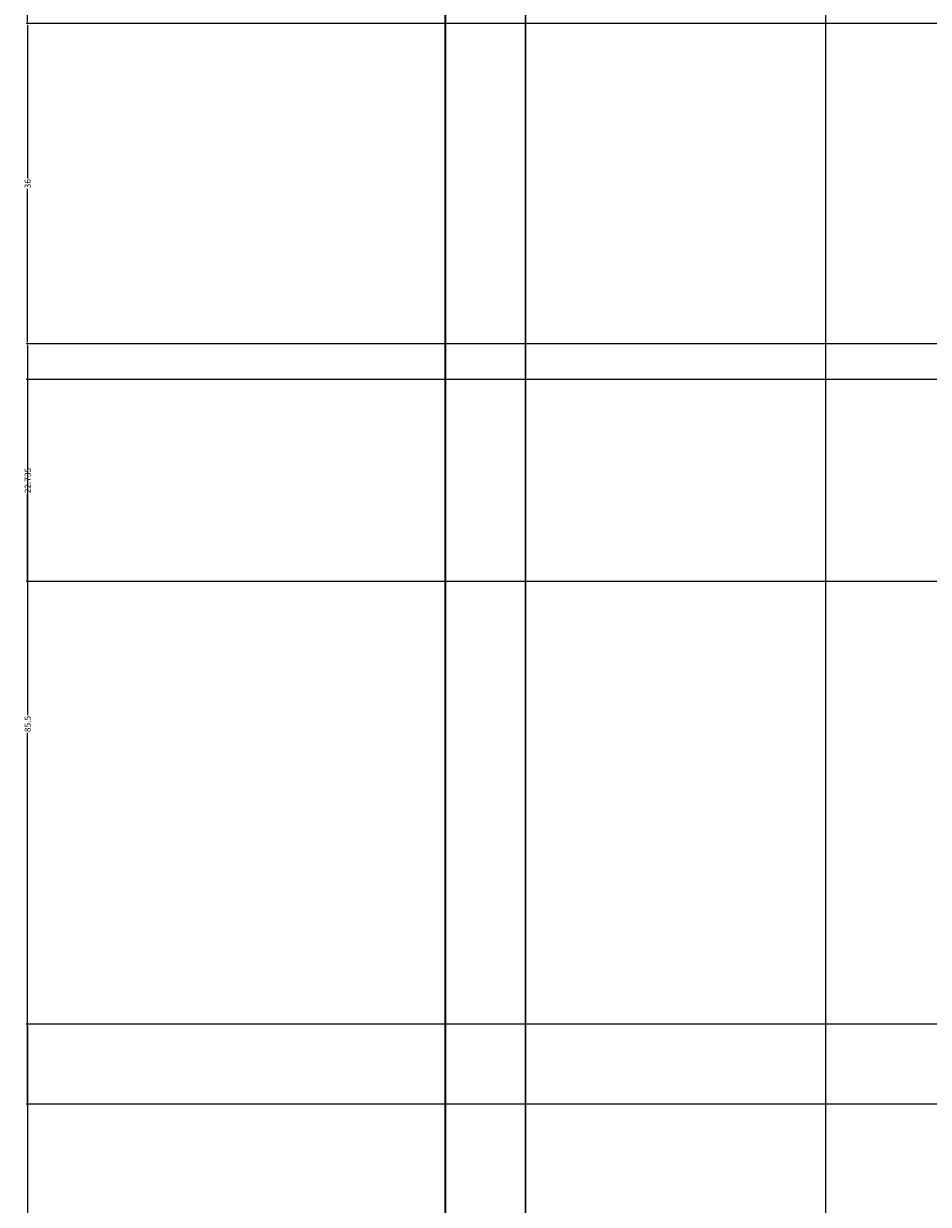
# Model space of a CAD drawing. Units: inches. Extents: x 867 to 1667, y -234 to 788.
# Tile 9 of 42: x 867 to 969, y 125 to 258. Entities that reach past the tile are written whole.
import ezdxf

# ---------------------------------------------------------------- set-up
doc = ezdxf.new("R2010")
doc.units = ezdxf.units.IN
doc.header["$MEASUREMENT"] = 0
doc.layers.add('A-ANNO-DIMS', color=2, linetype='Continuous', lineweight=18)
doc.layers.add('A-WALL-SITE', color=8, linetype='Continuous', lineweight=30)
doc.styles.get("Standard").update_dxf_attribs({"font": 'arial.ttf'})
doc.dimstyles.get("Standard").update_dxf_attribs({"dimtxt": 0.6875, "dimasz": 0.18, "dimexe": 0.18, "dimexo": 0.0625, "dimgap": 0.09, "dimtad": 0, "dimdec": 4, "dimzin": 0, "dimdsep": 46, "dimlunit": 4, "dimtxsty": 'Standard', "dimcen": 0.09, "dimadec": 0, "dimazin": 0, "dimtfac": 1, "dimtdec": 4, "dimtofl": 0, "dimtmove": 0, "dimatfit": 3, "dimfxl": 1, "dimtolj": 1, "dimtzin": 0, "dimarcsym": 0})

# ---------------------------------------------------------------- blocks, each defined once
blk = doc.blocks.new('*D28')
at = {"layer": 'A-ANNO-DIMS', "color": 0, "lineweight": -2, "transparency": 16777216}
for p, q in [((914.89, 623.55), (914.89, -233.54)), ((957.64, 623.55), (957.64, -233.54)), ((915.07, -233.36), (935, -233.36)), ((957.46, -233.36), (937.53, -233.36))]:
    blk.add_line(p, q, dxfattribs=at)
at = {"layer": 'A-ANNO-DIMS', "color": 0, "transparency": 16777216}
for points in [[(915.07, -233.33), (915.07, -233.39), (914.89, -233.36)], [(957.46, -233.33), (957.46, -233.39), (957.64, -233.36)]]:
    blk.add_solid(points, dxfattribs=at)
at = {"layer": 'Defpoints', "color": 0, "transparency": 16777216}
for p in [(914.89, 623.62), (957.64, 623.62), (914.89, -233.36)]:
    blk.add_point(p, dxfattribs=at)
at = {"layer": 'A-ANNO-DIMS', "color": 0, "transparency": 16777216, "insert": (936.26, -233.36), "char_height": 0.688, "attachment_point": 5}
blk.add_mtext('\\A1;42.75', dxfattribs=at)
blk = doc.blocks.new('*D39')
at = {"layer": 'A-ANNO-DIMS', "color": 0, "lineweight": -2, "transparency": 16777216}
for p, q in [((1040.82, 413.62), (867.76, 413.62)), ((867.94, 413.44), (867.94, 336.43)), ((867.94, 257.8), (867.94, 334.8)), ((1040.82, 257.62), (867.76, 257.62))]:
    blk.add_line(p, q, dxfattribs=at)
at = {"layer": 'A-ANNO-DIMS', "color": 0, "transparency": 16777216}
for points in [[(867.91, 413.44), (867.97, 413.44), (867.94, 413.62)], [(867.91, 257.8), (867.97, 257.8), (867.94, 257.62)]]:
    blk.add_solid(points, dxfattribs=at)
at = {"layer": 'Defpoints', "color": 0, "transparency": 16777216}
for p in [(867.94, 413.62), (1040.89, 413.62), (1040.89, 257.62)]:
    blk.add_point(p, dxfattribs=at)
at = {"layer": 'A-ANNO-DIMS', "color": 0, "transparency": 16777216, "insert": (867.94, 335.62), "char_height": 0.688, "attachment_point": 5, "rotation": 90}
blk.add_mtext('\\A1;156', dxfattribs=at)
blk = doc.blocks.new('*D40')
at = {"layer": 'A-ANNO-DIMS', "color": 0, "lineweight": -2, "transparency": 16777216}
for p, q in [((1040.82, 257.62), (867.76, 257.62)), ((867.94, 257.44), (867.94, 240.2)), ((867.94, 221.8), (867.94, 239.04)), ((1070.82, 221.62), (867.76, 221.62))]:
    blk.add_line(p, q, dxfattribs=at)
at = {"layer": 'A-ANNO-DIMS', "color": 0, "transparency": 16777216}
for points in [[(867.91, 257.44), (867.97, 257.44), (867.94, 257.62)], [(867.91, 221.8), (867.97, 221.8), (867.94, 221.62)]]:
    blk.add_solid(points, dxfattribs=at)
at = {"layer": 'Defpoints', "color": 0, "transparency": 16777216}
for p in [(1040.89, 257.62), (867.94, 221.62), (1070.89, 221.62)]:
    blk.add_point(p, dxfattribs=at)
at = {"layer": 'A-ANNO-DIMS', "color": 0, "transparency": 16777216, "insert": (867.94, 239.62), "char_height": 0.688, "attachment_point": 5, "rotation": 90}
blk.add_mtext('\\A1;36', dxfattribs=at)
blk = doc.blocks.new('*D41')
at = {"layer": 'A-ANNO-DIMS', "color": 0, "lineweight": -2, "transparency": 16777216}
for p, q in [((1149.82, 221.62), (867.76, 221.62)), ((867.94, 221.44), (867.94, 179.85)), ((867.94, 136.3), (867.94, 177.88)), ((1149.82, 136.12), (867.76, 136.12))]:
    blk.add_line(p, q, dxfattribs=at)
at = {"layer": 'A-ANNO-DIMS', "color": 0, "transparency": 16777216}
for points in [[(867.91, 221.44), (867.97, 221.44), (867.94, 221.62)], [(867.91, 136.3), (867.97, 136.3), (867.94, 136.12)]]:
    blk.add_solid(points, dxfattribs=at)
at = {"layer": 'Defpoints', "color": 0, "transparency": 16777216}
for p in [(867.94, 221.62), (1149.89, 221.62), (1149.89, 136.12)]:
    blk.add_point(p, dxfattribs=at)
at = {"layer": 'A-ANNO-DIMS', "color": 0, "transparency": 16777216, "insert": (867.94, 178.87), "char_height": 0.688, "attachment_point": 5, "rotation": 90}
blk.add_mtext('\\A1;85.5', dxfattribs=at)
blk = doc.blocks.new('*D44')
at = {"layer": 'A-ANNO-DIMS', "color": 0, "lineweight": -2, "transparency": 16777216}
for p, q in [((1070.82, 145.12), (867.76, 145.12)), ((867.94, 144.94), (867.94, 64.93)), ((867.94, -16.7), (867.94, 63.3)), ((1070.82, -16.88), (867.76, -16.88))]:
    blk.add_line(p, q, dxfattribs=at)
at = {"layer": 'A-ANNO-DIMS', "color": 0, "transparency": 16777216}
for points in [[(867.91, 144.94), (867.97, 144.94), (867.94, 145.12)], [(867.91, -16.7), (867.97, -16.7), (867.94, -16.88)]]:
    blk.add_solid(points, dxfattribs=at)
at = {"layer": 'Defpoints', "color": 0, "transparency": 16777216}
for p in [(867.94, 145.12), (1070.89, 145.12), (1070.89, -16.88)]:
    blk.add_point(p, dxfattribs=at)
at = {"layer": 'A-ANNO-DIMS', "color": 0, "transparency": 16777216, "insert": (867.94, 64.12), "char_height": 0.688, "attachment_point": 5, "rotation": 90}
blk.add_mtext('\\A1;162', dxfattribs=at)
blk = doc.blocks.new('*D56')
at = {"layer": 'A-ANNO-DIMS', "color": 0, "lineweight": -2, "transparency": 16777216}
for p, q in [((1049.82, 300.59), (867.76, 300.59)), ((867.94, 300.41), (867.94, 280.37)), ((867.94, 257.8), (867.94, 277.84)), ((1049.82, 257.62), (867.76, 257.62))]:
    blk.add_line(p, q, dxfattribs=at)
at = {"layer": 'A-ANNO-DIMS', "color": 0, "transparency": 16777216}
for points in [[(867.91, 300.41), (867.97, 300.41), (867.94, 300.59)], [(867.91, 257.8), (867.97, 257.8), (867.94, 257.62)]]:
    blk.add_solid(points, dxfattribs=at)
at = {"layer": 'Defpoints', "color": 0, "transparency": 16777216}
for p in [(867.94, 300.59), (1049.89, 300.59), (1049.89, 257.62)]:
    blk.add_point(p, dxfattribs=at)
at = {"layer": 'A-ANNO-DIMS', "color": 0, "transparency": 16777216, "insert": (867.94, 279.1), "char_height": 0.688, "attachment_point": 5, "rotation": 90}
blk.add_mtext('\\A1;42.97', dxfattribs=at)
blk = doc.blocks.new('*D61')
at = {"layer": 'A-ANNO-DIMS', "color": 0, "lineweight": -2, "transparency": 16777216}
for p, q in [((1076.39, 217.62), (867.76, 217.62)), ((867.94, 217.44), (867.94, 207.78)), ((867.94, 195.06), (867.94, 204.72)), ((1079.82, 194.88), (867.76, 194.88))]:
    blk.add_line(p, q, dxfattribs=at)
at = {"layer": 'A-ANNO-DIMS', "color": 0, "transparency": 16777216}
for points in [[(867.91, 217.44), (867.97, 217.44), (867.94, 217.62)], [(867.91, 195.06), (867.97, 195.06), (867.94, 194.88)]]:
    blk.add_solid(points, dxfattribs=at)
at = {"layer": 'Defpoints', "color": 0, "transparency": 16777216}
for p in [(867.94, 217.62), (1076.46, 217.62), (1079.89, 194.88)]:
    blk.add_point(p, dxfattribs=at)
at = {"layer": 'A-ANNO-DIMS', "color": 0, "transparency": 16777216, "insert": (867.94, 206.25), "char_height": 0.688, "attachment_point": 5, "rotation": 90}
blk.add_mtext('\\A1;22.735', dxfattribs=at)

msp = doc.modelspace()

# ---------------------------------------------------------------- linework, layer by layer
at = {"layer": 'A-WALL-SITE'}
for p, q in [((914.8866, 740.617), (914.8866, -186.4081)), ((923.8866, 740.617), (923.8866, -186.4081))]:
    msp.add_line(p, q, dxfattribs=at)

# ---------------------------------------------------------------- dimensions: what is measured, and where the dimension line sits
at = {"layer": 'A-ANNO-DIMS'}
dim = msp.add_linear_dim(base=(914.8866, -233.3581), p1=(957.6375, 623.617), p2=(914.8866, 623.617), dimstyle='Standard', override={"dimdec": 2, "dimlfac": 1, "dimrnd": 0, "dimzin": 0, "dimdsep": 46, "dimlunit": 2}, dxfattribs=at)
dim.commit()
dim.dimension.update_dxf_attribs({"geometry": '*D28', "text_midpoint": (936.2621, -233.3581)})
for base, p1, p2, override, picture, middle in [((867.9366, 413.617), (1040.8866, 257.617), (1040.8866, 413.617), {"dimdec": 0, "dimlfac": 1, "dimrnd": 0, "dimzin": 0, "dimdsep": 46, "dimlunit": 2}, '*D39', (867.9366, 335.617)), ((867.9366, 300.5856), (1049.8866, 257.617), (1049.8866, 300.5856), {"dimdec": 2, "dimlfac": 1, "dimrnd": 0, "dimzin": 0, "dimdsep": 46, "dimlunit": 2}, '*D56', (867.9366, 279.1013)), ((867.9366, 221.617), (1040.8866, 257.617), (1070.8866, 221.617), {"dimdec": 0, "dimlfac": 1, "dimrnd": 0, "dimzin": 0, "dimdsep": 46, "dimlunit": 2}, '*D40', (867.9366, 239.617)), ((867.9366, 221.617), (1149.8866, 136.117), (1149.8866, 221.617), {"dimdec": 1, "dimlfac": 1, "dimrnd": 0, "dimzin": 0, "dimdsep": 46, "dimlunit": 2}, '*D41', (867.9366, 178.867)), ((867.9366, 217.617), (1079.8866, 194.8824), (1076.4575, 217.617), {"dimdec": 3, "dimlfac": 1, "dimrnd": 0, "dimzin": 0, "dimdsep": 46, "dimlunit": 2}, '*D61', (867.9366, 206.2497)), ((867.9366, 145.117), (1070.8866, -16.883), (1070.8866, 145.117), {"dimdec": 0, "dimlfac": 1, "dimrnd": 0, "dimzin": 0, "dimdsep": 46, "dimlunit": 2}, '*D44', (867.9366, 64.117))]:
    dim = msp.add_linear_dim(base=base, p1=p1, p2=p2, angle=90, dimstyle='Standard', override=override, dxfattribs=at)
    dim.commit()
    dim.dimension.update_dxf_attribs({"geometry": picture, "text_midpoint": middle})

doc.saveas('drawing.dxf')
